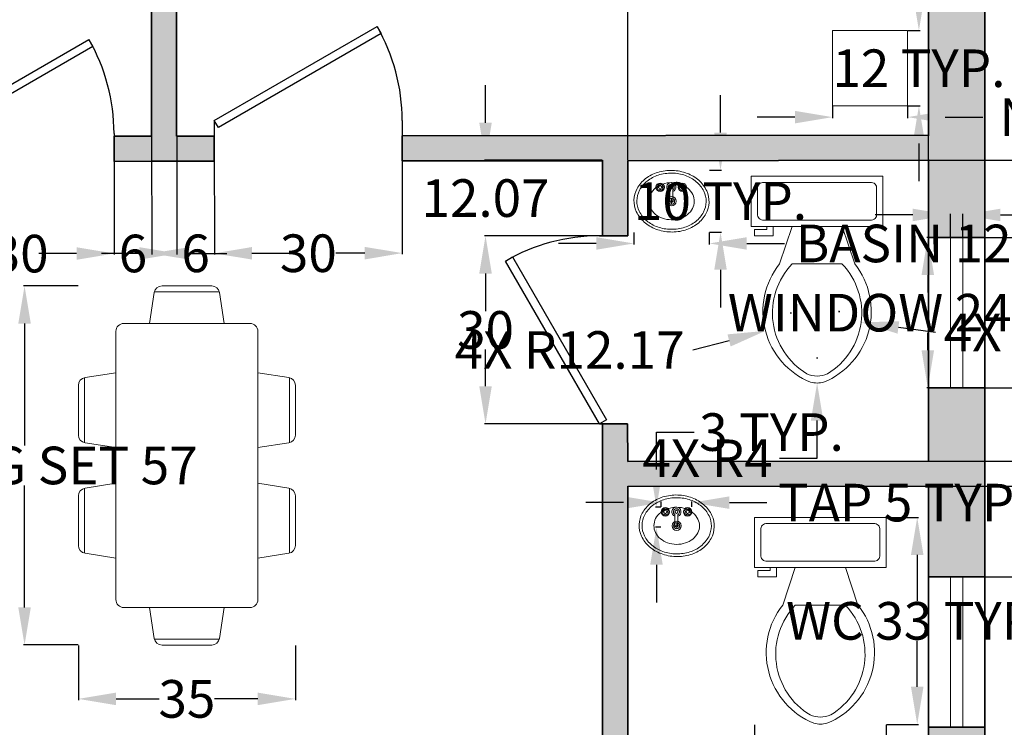
# Model space of a CAD drawing. Units: inches. Extents: x 98 to 487, y -240 to 141.
# Tile 3 of 5: x 251 to 408, y -81 to 32. Entities that reach past the tile are written whole.
import ezdxf

# ---------------------------------------------------------------- set-up
doc = ezdxf.new("R2010")
doc.units = ezdxf.units.IN
doc.header["$MEASUREMENT"] = 0
for name, color, linetype, lineweight in [('A-ANNO-DIMS', 2, 'Continuous', 18), ('A-DOOR', 3, 'Continuous', 25), ('A-FLOR-FIXT', 9, 'Continuous', 18), ('A-FURN', 8, 'Continuous', 18), ('A-GLAZ', 4, 'Continuous', 18), ('A-WALL', 7, 'Continuous', 35)]:
    doc.layers.add(name, color=color, linetype=linetype, lineweight=lineweight)
doc.layers.add('A-WALL-PATT', color=251, linetype='Continuous', lineweight=13, true_color=0x636466)
doc.styles.get("Standard").update_dxf_attribs({"font": 'arial.ttf'})
doc.dimstyles.get("Standard").update_dxf_attribs({"dimtxt": 6, "dimasz": 6, "dimexe": 0.18, "dimexo": 0.0625, "dimgap": 0.09, "dimtad": 0, "dimtih": 1, "dimtoh": 1, "dimdec": 0, "dimzin": 0, "dimdsep": 46, "dimlunit": 4, "dimtxsty": 'Standard', "dimcen": 0.09, "dimadec": 0, "dimazin": 0, "dimtfac": 1, "dimtdec": 0, "dimtofl": 0, "dimtmove": 0, "dimatfit": 3, "dimfxl": 1, "dimtolj": 1, "dimtzin": 0, "dimarcsym": 0})

# ---------------------------------------------------------------- blocks, each defined once
blk = doc.blocks.new('Sink - Oval top')
for p, q in [((-1, 0), (1, 0)), ((0, 1), (0, -1))]:
    blk.add_line(p, q)
for points in [[(-12.23, 0.39, 0.117634), (-11.46, -3.36, 0.104469), (-8.88, -6.8, 0.090016), (-5.08, -9.07, 0.08192), (-0.32, -10.02, 0.08192), (4.49, -9.38, 0.090016), (8.42, -7.36, 0.104469), (11.22, -4.09, 0.117634), (12.23, -0.39, 0.117634), (11.46, 3.36, 0.104469), (8.88, 6.8, 0.090016), (5.08, 9.07, 0.08192), (0.32, 10.02, 0.08192), (-4.49, 9.38, 0.090016), (-8.42, 7.36, 0.104469), (-11.22, 4.09, 0.117634)], [(-11.29, 0.16, 0.118622), (-10.52, -3.25, 0.104678), (-8.07, -6.36, 0.089562), (-4.54, -8.37, 0.081185), (-0.13, -9.15, 0.081185), (4.3, -8.49, 0.089562), (7.89, -6.58, 0.104678), (10.42, -3.55, 0.118622), (11.29, -0.16, 0.118622), (10.52, 3.25, 0.104678), (8.07, 6.36, 0.089562), (4.54, 8.37, 0.081185), (0.13, 9.15, 0.081185), (-4.3, 8.49, 0.089562), (-7.89, 6.58, 0.104678), (-10.42, 3.55, 0.118622)], [(-7.42, 0.08, 0.118283), (-6.91, -2.17, 0.104607), (-5.29, -4.21, 0.089718), (-2.97, -5.53, 0.081436), (-0.07, -6.04, 0.081436), (2.84, -5.59, 0.089718), (5.2, -4.33, 0.104607), (6.86, -2.32, 0.118283), (7.42, -0.08, 0.118283), (6.91, 2.17, 0.104607), (5.29, 4.21, 0.089718), (2.97, 5.53, 0.081436), (0.07, 6.04, 0.081436), (-2.84, 5.59, 0.089718), (-5.2, 4.33, 0.104607), (-6.86, 2.32, 0.118283)]]:
    blk.add_lwpolyline(points, format="xyb", close=True)
for radius in [1.5, 1]:
    blk.add_circle((0, 0), radius)
blk = doc.blocks.new('Faucet - Bathroom top')
for p, q in [((-4.107, 0.125), (-4.375, 0.125)), ((-3.75, 0.4788), (-3.75, 0.75)), ((-3.5, 0.482), (-3.5, 0.75)), ((-3.1461, 0.125), (-2.875, 0.125)), ((3.143, 0.125), (2.875, 0.125)), ((3.5, 0.4788), (3.5, 0.75)), ((3.75, 0.482), (3.75, 0.75)), ((4.1039, 0.125), (4.375, 0.125)), ((-4.1039, -0.125), (-4.375, -0.125)), ((-3.75, -0.4821), (-3.75, -0.75)), ((-3.5, -0.4789), (-3.5, -0.75)), ((-3.143, -0.125), (-2.875, -0.125)), ((-0.5, -0.8639), (-0.5, -4.5)), ((0.5, -4.5), (0.5, -0.8631)), ((3.1461, -0.125), (2.875, -0.125)), ((3.5, -0.4821), (3.5, -0.75)), ((3.75, -0.4789), (3.75, -0.75)), ((4.107, -0.125), (4.375, -0.125))]:
    blk.add_line(p, q)
for centre, radius in [((-3.625, 0), 1.375), ((-4.625, 0), 0.2795), ((-3.625, 0), 0.5), ((-3.625, 1), 0.2795), ((-2.625, 0), 0.2795), ((0, 0), 0.5), ((3.625, 0), 1.375), ((2.625, 0), 0.2795), ((3.625, 0), 0.5), ((3.625, 1), 0.2795), ((4.625, 0), 0.2795), ((-3.625, -1), 0.2795), ((3.625, -1), 0.2795)]:
    blk.add_circle(centre, radius)
for centre, radius, start, end in [((-3.625, 0), 1, 105.2407, 164.2093), ((-3.625, 0), 1, 16.44125, 74.07887), ((0, 0), 1.5, 289.6514, 250.3603), ((0, 0), 1, 300.3431, 239.7554), ((3.625, 0), 1, 106.12, 164.0884), ((3.625, 0), 1, 16.23422, 73.90469), ((-3.625, 0), 1, 196.2342, 253.9047), ((-3.625, 0), 1, 286.12, 344.0884), ((3.625, 0), 1, 196.4413, 254.0789), ((3.625, 0), 1, 285.2407, 344.2093), ((0, -4.5), 0.5, 180, 0)]:
    blk.add_arc(centre, radius, start, end)
blk = doc.blocks.new('Toilet - top')
for p, q in [((9.5, -6), (9.5, -2)), ((-10, -8.5), (-8, -8.5)), ((-10, -9.5), (-10, -8.5)), ((-8, -8.5), (-8, -8)), ((-7, -8), (-7, -9.5)), ((-4, -8), (-6, -14)), ((4, -8), (6, -14)), ((-7, -9.5), (-10, -9.5)), ((4, -14), (-4, -14))]:
    blk.add_line(p, q)
blk.add_lwpolyline([(10.5, -8), (10.5, 0), (-10.5, 0), (-10.5, -8)], close=True)
for points in [[(8.5, -1), (-8.5, -1)], [(-9.5, -2), (-9.5, -6)], [(-8.5, -7), (8.5, -7)]]:
    blk.add_lwpolyline(points)
for centre, radius, start, end in [((-8.62, -1.88), 0.884, 81.8699, 188.1301), ((8.62, -1.88), 0.884, 351.8699, 98.1301), ((-8.62, -6.12), 0.884, 171.8699, 278.1301), ((8.62, -6.12), 0.884, 261.8699, 8.1301), ((3.52, -21.58), 12.17, 141.4691, 247.9714), ((4.2, -21.82), 11.33, 136.3677, 238.9468), ((-3.52, -21.58), 12.17, 292.0284, 38.5307), ((-4.2, -21.82), 11.33, 301.053, 43.6321), ((0, -27.88), 4, 245.7318, 294.2682), ((0, -29), 4, 254.8605, 285.1395)]:
    blk.add_arc(centre, radius, start, end)
blk = doc.blocks.new('Dining Set - 36 x 72 in.')
for p, q in [((-20.29, 27.5), (-7.71, 27.5)), ((7.71, 27.5), (20.29, 27.5)), ((-22.26, 25.81), (-23.48, 18)), ((-22.23, 26), (-5.76, 26)), ((-4.52, 18), (-5.74, 25.81)), ((5.74, 25.81), (4.52, 18)), ((5.77, 26), (22.24, 26)), ((23.48, 18), (22.26, 25.81)), ((34, 18), (-34, 18)), ((-36, 16), (-36, -16)), ((36, -16), (36, 16)), ((-44, 8.23), (-44, -8.24)), ((-43.81, 8.26), (-36, 9.48)), ((43.81, 8.26), (36, 9.48)), ((44, 8.23), (44, -8.24)), ((-45.5, 6.29), (-45.5, -6.29)), ((45.5, 6.29), (45.5, -6.29)), ((-36, -9.48), (-43.81, -8.26)), ((36, -9.48), (43.81, -8.26)), ((-34, -18), (34, -18)), ((-22.26, -25.81), (-23.48, -18)), ((-4.52, -18), (-5.74, -25.81)), ((5.74, -25.81), (4.52, -18)), ((23.48, -18), (22.26, -25.81)), ((-22.23, -26), (-5.76, -26)), ((5.77, -26), (22.24, -26)), ((-20.29, -27.5), (-7.71, -27.5)), ((7.71, -27.5), (20.29, -27.5))]:
    blk.add_line(p, q)
for centre, start, end in [((-20.29, 25.5), 90, 171.1198), ((-7.71, 25.5), 8.881, 90), ((7.71, 25.5), 90, 171.1198), ((20.29, 25.5), 8.881, 90), ((-34, 16), 90, 180), ((34, 16), 0, 90), ((-43.5, 6.29), 98.8806, 180), ((43.5, 6.29), 0, 81.1194), ((-43.5, -6.29), 180, 261.1194), ((43.5, -6.29), 278.8806, 0), ((-34, -16), 180, 270), ((34, -16), 270, 0), ((-20.29, -25.5), 188.8802, 270), ((-7.71, -25.5), 270, 351.1191), ((7.71, -25.5), 188.8802, 270), ((20.29, -25.5), 270, 351.1191)]:
    blk.add_arc(centre, 2, start, end)
blk = doc.blocks.new('*U8')
for p, q in [((0, 0), (0, -6)), ((40, 0), (40, -6))]:
    blk.add_line(p, q)
blk.add_lwpolyline([(0, 0), (34.64, 20), (35.52, 18.48), (0.87, -1.52)], close=True)
blk.add_arc((0, 0), 40, 0, 30)
blk = doc.blocks.new('GLAZ-24IN')
for p, q in [((0, 24), (0, 0)), ((2, 24), (2, 0))]:
    blk.add_line(p, q)
blk = doc.blocks.new('NIGHTSTAND-12IN-SQUARE')
blk.add_lwpolyline([(12, 12), (0, 12), (0, 0), (12, 0)], close=True)
blk = doc.blocks.new('*D26')
at = {"layer": 'A-ANNO-DIMS', "color": 0, "lineweight": -2, "transparency": 16777216}
for p, q in [((380.45, 18.25), (380.45, 16.33)), ((392.45, 18.25), (392.45, 16.33)), ((374.45, 16.51), (368.45, 16.51)), ((398.45, 16.51), (404.45, 16.51))]:
    blk.add_line(p, q, dxfattribs=at)
at = {"layer": 'A-ANNO-DIMS', "color": 0, "transparency": 16777216}
for points in [[(374.45, 17.51), (374.45, 15.51), (380.45, 16.51)], [(398.45, 17.51), (398.45, 15.51), (392.45, 16.51)]]:
    blk.add_solid(points, dxfattribs=at)
at = {"layer": 'Defpoints', "color": 0, "transparency": 16777216}
for p in [(380.45, 18.31), (392.45, 18.31), (392.45, 16.51)]:
    blk.add_point(p, dxfattribs=at)
at = {"layer": 'A-ANNO-DIMS', "color": 0, "transparency": 16777216, "insert": (447.4, 16.51), "char_height": 6, "attachment_point": 5}
blk.add_mtext('\\A1;NIGHTSTAND 12 TYP.', dxfattribs=at)
blk = doc.blocks.new('*D27')
at = {"layer": 'A-ANNO-DIMS', "color": 0, "lineweight": -2, "transparency": 16777216}
for p, q in [((394.25, 36.31), (394.25, 42.31)), ((392.51, 30.31), (394.43, 30.31)), ((392.51, 18.31), (394.43, 18.31)), ((394.25, 12.31), (394.25, 6.31))]:
    blk.add_line(p, q, dxfattribs=at)
at = {"layer": 'A-ANNO-DIMS', "color": 0, "transparency": 16777216}
for points in [[(393.25, 36.31), (395.25, 36.31), (394.25, 30.31)], [(393.25, 12.31), (395.25, 12.31), (394.25, 18.31)]]:
    blk.add_solid(points, dxfattribs=at)
at = {"layer": 'Defpoints', "color": 0, "transparency": 16777216}
for p in [(392.45, 30.31), (394.25, 30.31), (392.45, 18.31)]:
    blk.add_point(p, dxfattribs=at)
at = {"layer": 'A-ANNO-DIMS', "color": 0, "transparency": 16777216, "insert": (394.25, 24.31), "char_height": 6, "attachment_point": 5}
blk.add_mtext('\\A1;12 TYP.', dxfattribs=at)
blk = doc.blocks.new('*D30')
at = {"layer": 'A-ANNO-DIMS', "color": 0, "lineweight": -2, "transparency": 16777216}
for p, q in [((399.2, -2.7), (395.49, -2.7)), ((395.67, -8.7), (395.67, -11.5)), ((395.67, -20.7), (395.67, -17.89)), ((399.2, -26.7), (395.49, -26.7))]:
    blk.add_line(p, q, dxfattribs=at)
at = {"layer": 'A-ANNO-DIMS', "color": 0, "transparency": 16777216}
for points in [[(394.67, -8.7), (396.67, -8.7), (395.67, -2.7)], [(394.67, -20.7), (396.67, -20.7), (395.67, -26.7)]]:
    blk.add_solid(points, dxfattribs=at)
at = {"layer": 'Defpoints', "color": 0, "transparency": 16777216}
for p in [(395.67, -2.7), (399.27, -2.7), (399.27, -26.7)]:
    blk.add_point(p, dxfattribs=at)
at = {"layer": 'A-ANNO-DIMS', "color": 0, "transparency": 16777216, "insert": (395.67, -14.7), "char_height": 6, "attachment_point": 5}
blk.add_mtext('\\A1;WINDOW 24 TYP.', dxfattribs=at)
blk = doc.blocks.new('*D31')
at = {"layer": 'A-ANNO-DIMS', "color": 0, "lineweight": -2, "transparency": 16777216}
for p, q in [((393.27, 0.9), (387.27, 0.9)), ((399.27, -2.64), (399.27, 1.08)), ((401.27, -2.64), (401.27, 1.08)), ((407.27, 0.9), (413.27, 0.9))]:
    blk.add_line(p, q, dxfattribs=at)
at = {"layer": 'A-ANNO-DIMS', "color": 0, "transparency": 16777216}
for points in [[(393.27, 1.9), (393.27, -0.1), (399.27, 0.9)], [(407.27, 1.9), (407.27, -0.1), (401.27, 0.9)]]:
    blk.add_solid(points, dxfattribs=at)
at = {"layer": 'Defpoints', "color": 0, "transparency": 16777216}
for p in [(401.27, 0.9), (399.27, -2.7), (401.27, -2.7)]:
    blk.add_point(p, dxfattribs=at)
at = {"layer": 'A-ANNO-DIMS', "color": 0, "transparency": 16777216, "insert": (425.68, 0.9), "char_height": 6, "attachment_point": 5}
blk.add_mtext('\\A1;2 TYP.', dxfattribs=at)
blk = doc.blocks.new('*D32')
at = {"layer": 'A-ANNO-DIMS', "color": 0, "lineweight": -2, "transparency": 16777216}
for p, q in [((348.74, -1.91), (348.74, -3.83)), ((360.78, -1.91), (360.78, -3.83)), ((342.74, -3.65), (336.74, -3.65)), ((366.78, -3.65), (372.78, -3.65))]:
    blk.add_line(p, q, dxfattribs=at)
at = {"layer": 'A-ANNO-DIMS', "color": 0, "transparency": 16777216}
for points in [[(342.74, -2.65), (342.74, -4.65), (348.74, -3.65)], [(366.78, -2.65), (366.78, -4.65), (360.78, -3.65)]]:
    blk.add_solid(points, dxfattribs=at)
at = {"layer": 'Defpoints', "color": 0, "transparency": 16777216}
for p in [(348.74, -1.85), (360.78, -1.85), (360.78, -3.65)]:
    blk.add_point(p, dxfattribs=at)
at = {"layer": 'A-ANNO-DIMS', "color": 0, "transparency": 16777216, "insert": (401.08, -3.65), "char_height": 6, "attachment_point": 5}
blk.add_mtext('\\A1;BASIN 12 TYP.', dxfattribs=at)
blk = doc.blocks.new('*D33')
at = {"layer": 'A-ANNO-DIMS', "color": 0, "lineweight": -2, "transparency": 16777216}
for p, q in [((362.58, 14.03), (362.58, 20.03)), ((360.84, 8.03), (362.76, 8.03)), ((360.84, -1.85), (362.76, -1.85)), ((362.58, -7.85), (362.58, -13.85))]:
    blk.add_line(p, q, dxfattribs=at)
at = {"layer": 'A-ANNO-DIMS', "color": 0, "transparency": 16777216}
for points in [[(361.58, 14.03), (363.58, 14.03), (362.58, 8.03)], [(361.58, -7.85), (363.58, -7.85), (362.58, -1.85)]]:
    blk.add_solid(points, dxfattribs=at)
at = {"layer": 'Defpoints', "color": 0, "transparency": 16777216}
for p in [(360.78, 8.03), (362.58, 8.03), (360.78, -1.85)]:
    blk.add_point(p, dxfattribs=at)
at = {"layer": 'A-ANNO-DIMS', "color": 0, "transparency": 16777216, "insert": (362.58, 3.09), "char_height": 6, "attachment_point": 5}
blk.add_mtext('\\A1;10 TYP.', dxfattribs=at)
blk = doc.blocks.new('*D34')
at = {"layer": 'A-ANNO-DIMS', "color": 0, "lineweight": -2, "transparency": 16777216}
for p, q in [((347.1, -45.01), (341.1, -45.01)), ((353.1, -45.68), (353.1, -44.83)), ((358, -45.68), (358, -44.83)), ((364, -45.01), (370, -45.01))]:
    blk.add_line(p, q, dxfattribs=at)
at = {"layer": 'A-ANNO-DIMS', "color": 0, "transparency": 16777216}
for points in [[(347.1, -44.01), (347.1, -46.01), (353.1, -45.01)], [(364, -44.01), (364, -46.01), (358, -45.01)]]:
    blk.add_solid(points, dxfattribs=at)
at = {"layer": 'Defpoints', "color": 0, "transparency": 16777216}
for p in [(358, -45.01), (353.1, -45.75), (358, -45.75)]:
    blk.add_point(p, dxfattribs=at)
at = {"layer": 'A-ANNO-DIMS', "color": 0, "transparency": 16777216, "insert": (391.75, -45.01), "char_height": 6, "attachment_point": 5}
blk.add_mtext('\\A1;TAP 5 TYP.', dxfattribs=at)
blk = doc.blocks.new('*D35')
at = {"layer": 'A-ANNO-DIMS', "color": 0, "lineweight": -2, "transparency": 16777216}
for p, q in [((352.36, -39.75), (352.36, -33.75)), ((352.36, -33.75), (358.36, -33.75)), ((353.03, -45.75), (352.18, -45.75)), ((353.03, -48.93), (352.18, -48.93)), ((352.36, -54.93), (352.36, -60.93))]:
    blk.add_line(p, q, dxfattribs=at)
at = {"layer": 'A-ANNO-DIMS', "color": 0, "transparency": 16777216}
for points in [[(351.36, -39.75), (353.36, -39.75), (352.36, -45.75)], [(351.36, -54.93), (353.36, -54.93), (352.36, -48.93)]]:
    blk.add_solid(points, dxfattribs=at)
at = {"layer": 'Defpoints', "color": 0, "transparency": 16777216}
for p in [(352.36, -45.75), (353.1, -45.75), (353.1, -48.93)]:
    blk.add_point(p, dxfattribs=at)
at = {"layer": 'A-ANNO-DIMS', "color": 0, "transparency": 16777216, "insert": (370.72, -33.75), "char_height": 6, "attachment_point": 5}
blk.add_mtext('\\A1;3 TYP.', dxfattribs=at)
blk = doc.blocks.new('*D36')
at = {"layer": 'A-ANNO-DIMS', "color": 0, "lineweight": -2, "transparency": 16777216}
for p, q in [((389.08, -47.36), (394.16, -47.36)), ((393.98, -53.36), (393.98, -60.69)), ((393.98, -74.4), (393.98, -67.08)), ((389.08, -80.4), (394.16, -80.4))]:
    blk.add_line(p, q, dxfattribs=at)
at = {"layer": 'A-ANNO-DIMS', "color": 0, "transparency": 16777216}
for points in [[(392.98, -53.36), (394.98, -53.36), (393.98, -47.36)], [(392.98, -74.4), (394.98, -74.4), (393.98, -80.4)]]:
    blk.add_solid(points, dxfattribs=at)
at = {"layer": 'Defpoints', "color": 0, "transparency": 16777216}
for p in [(389.02, -47.36), (393.98, -47.36), (389.02, -80.4)]:
    blk.add_point(p, dxfattribs=at)
at = {"layer": 'A-ANNO-DIMS', "color": 0, "transparency": 16777216, "insert": (393.98, -63.88), "char_height": 6, "attachment_point": 5}
blk.add_mtext('\\A1;WC 33 TYP.', dxfattribs=at)
blk = doc.blocks.new('*D37')
at = {"layer": 'A-ANNO-DIMS', "color": 0, "lineweight": -2, "transparency": 16777216}
for p, q in [((368.02, -80.47), (368.02, -85.54)), ((389.02, -80.47), (389.02, -85.54)), ((374.02, -85.36), (383.02, -85.36)), ((389.02, -85.36), (395.02, -85.36))]:
    blk.add_line(p, q, dxfattribs=at)
at = {"layer": 'A-ANNO-DIMS', "color": 0, "transparency": 16777216}
for points in [[(374.02, -84.36), (374.02, -86.36), (368.02, -85.36)], [(383.02, -84.36), (383.02, -86.36), (389.02, -85.36)]]:
    blk.add_solid(points, dxfattribs=at)
at = {"layer": 'Defpoints', "color": 0, "transparency": 16777216}
for p in [(368.02, -80.4), (389.02, -80.4), (389.02, -85.36)]:
    blk.add_point(p, dxfattribs=at)
at = {"layer": 'A-ANNO-DIMS', "color": 0, "transparency": 16777216, "insert": (409.76, -85.36), "char_height": 6, "attachment_point": 5}
blk.add_mtext('\\A1;21 TYP.', dxfattribs=at)
blk = doc.blocks.new('*D38')
at = {"layer": 'A-ANNO-DIMS', "color": 0, "lineweight": -2, "transparency": 16777216}
for p, q in [((260.02, -10.43), (251.31, -10.43)), ((251.49, -16.43), (251.49, -35.89)), ((251.49, -61.73), (251.49, -42.27)), ((260.02, -67.73), (251.31, -67.73))]:
    blk.add_line(p, q, dxfattribs=at)
at = {"layer": 'A-ANNO-DIMS', "color": 0, "transparency": 16777216}
for points in [[(250.49, -16.43), (252.49, -16.43), (251.49, -10.43)], [(250.49, -61.73), (252.49, -61.73), (251.49, -67.73)]]:
    blk.add_solid(points, dxfattribs=at)
at = {"layer": 'Defpoints', "color": 0, "transparency": 16777216}
for p in [(260.09, -10.43), (251.49, -67.73), (260.09, -67.73)]:
    blk.add_point(p, dxfattribs=at)
at = {"layer": 'A-ANNO-DIMS', "color": 0, "transparency": 16777216, "insert": (251.49, -39.08), "char_height": 6, "attachment_point": 5}
blk.add_mtext('\\A1;DINING SET 57', dxfattribs=at)
blk = doc.blocks.new('*D39')
at = {"layer": 'A-ANNO-DIMS', "color": 0, "lineweight": -2, "transparency": 16777216}
for p, q in [((260.09, -67.8), (260.09, -76.51)), ((294.72, -67.8), (294.72, -76.51)), ((266.09, -76.33), (273, -76.33)), ((288.72, -76.33), (281.81, -76.33))]:
    blk.add_line(p, q, dxfattribs=at)
at = {"layer": 'A-ANNO-DIMS', "color": 0, "transparency": 16777216}
for points in [[(266.09, -75.33), (266.09, -77.33), (260.09, -76.33)], [(288.72, -75.33), (288.72, -77.33), (294.72, -76.33)]]:
    blk.add_solid(points, dxfattribs=at)
at = {"layer": 'Defpoints', "color": 0, "transparency": 16777216}
for p in [(260.09, -67.73), (294.72, -67.73), (294.72, -76.33)]:
    blk.add_point(p, dxfattribs=at)
at = {"layer": 'A-ANNO-DIMS', "color": 0, "transparency": 16777216, "insert": (277.4, -76.33), "char_height": 6, "attachment_point": 5}
blk.add_mtext('\\A1;35', dxfattribs=at)
blk = doc.blocks.new('*D47')
at = {"layer": 'A-ANNO-DIMS', "color": 0, "lineweight": -2, "transparency": 16777216}
for p, q in [((404.83, 118.64), (423.65, 118.64)), ((423.47, 112.64), (423.47, -46.22)), ((423.47, -211.38), (423.47, -52.53)), ((404.83, -217.38), (423.65, -217.38))]:
    blk.add_line(p, q, dxfattribs=at)
at = {"layer": 'A-ANNO-DIMS', "color": 0, "transparency": 16777216}
for points in [[(422.47, 112.64), (424.47, 112.64), (423.47, 118.64)], [(422.47, -211.38), (424.47, -211.38), (423.47, -217.38)]]:
    blk.add_solid(points, dxfattribs=at)
at = {"layer": 'Defpoints', "color": 0, "transparency": 16777216}
for p in [(404.77, 118.64), (404.77, -217.38), (423.47, -217.38)]:
    blk.add_point(p, dxfattribs=at)
at = {"layer": 'A-ANNO-DIMS', "color": 0, "transparency": 16777216, "insert": (423.47, -49.37), "char_height": 6, "attachment_point": 5}
blk.add_mtext('\\A1;336', dxfattribs=at)
blk = doc.blocks.new('*D65')
at = {"layer": 'A-ANNO-DIMS', "color": 0, "lineweight": -2, "transparency": 16777216}
for p, q in [((395.83, 9.62), (414.65, 9.62)), ((414.47, 3.62), (414.47, -11.22)), ((414.47, -32.38), (414.47, -17.53)), ((395.83, -38.38), (414.65, -38.38))]:
    blk.add_line(p, q, dxfattribs=at)
at = {"layer": 'A-ANNO-DIMS', "color": 0, "transparency": 16777216}
for points in [[(413.47, 3.62), (415.47, 3.62), (414.47, 9.62)], [(413.47, -32.38), (415.47, -32.38), (414.47, -38.38)]]:
    blk.add_solid(points, dxfattribs=at)
at = {"layer": 'Defpoints', "color": 0, "transparency": 16777216}
for p in [(395.77, 9.62), (395.77, -38.38), (414.47, -38.38)]:
    blk.add_point(p, dxfattribs=at)
at = {"layer": 'A-ANNO-DIMS', "color": 0, "transparency": 16777216, "insert": (414.47, -14.38), "char_height": 6, "attachment_point": 5}
blk.add_mtext('\\A1;48', dxfattribs=at)
blk = doc.blocks.new('*D66')
at = {"layer": 'A-ANNO-DIMS', "color": 0, "lineweight": -2, "transparency": 16777216}
for p, q in [((395.83, -42.38), (414.65, -42.38)), ((414.47, -48.38), (414.47, -63.22)), ((414.47, -84.38), (414.47, -69.53)), ((395.83, -90.38), (414.65, -90.38))]:
    blk.add_line(p, q, dxfattribs=at)
at = {"layer": 'A-ANNO-DIMS', "color": 0, "transparency": 16777216}
for points in [[(413.47, -48.38), (415.47, -48.38), (414.47, -42.38)], [(413.47, -84.38), (415.47, -84.38), (414.47, -90.38)]]:
    blk.add_solid(points, dxfattribs=at)
at = {"layer": 'Defpoints', "color": 0, "transparency": 16777216}
for p in [(395.77, -42.38), (395.77, -90.38), (414.47, -90.38)]:
    blk.add_point(p, dxfattribs=at)
at = {"layer": 'A-ANNO-DIMS', "color": 0, "transparency": 16777216, "insert": (414.47, -66.38), "char_height": 6, "attachment_point": 5}
blk.add_mtext('\\A1;48', dxfattribs=at)
blk = doc.blocks.new('*D67')
at = {"layer": 'A-ANNO-DIMS', "color": 0, "lineweight": -2, "transparency": 16777216}
for p, q in [((347.77, 9.62), (347.77, 137.52)), ((353.77, 137.34), (367.25, 137.34)), ((389.77, 137.34), (376.28, 137.34)), ((395.77, 9.69), (395.77, 137.52))]:
    blk.add_line(p, q, dxfattribs=at)
at = {"layer": 'A-ANNO-DIMS', "color": 0, "transparency": 16777216}
for points in [[(353.77, 138.34), (353.77, 136.34), (347.77, 137.34)], [(389.77, 138.34), (389.77, 136.34), (395.77, 137.34)]]:
    blk.add_solid(points, dxfattribs=at)
at = {"layer": 'Defpoints', "color": 0, "transparency": 16777216}
for p in [(395.77, 137.34), (347.77, 9.56), (395.77, 9.62)]:
    blk.add_point(p, dxfattribs=at)
at = {"layer": 'A-ANNO-DIMS', "color": 0, "transparency": 16777216, "insert": (371.77, 137.34), "char_height": 6, "attachment_point": 5}
blk.add_mtext('\\A1;48', dxfattribs=at)
blk = doc.blocks.new('*D70')
at = {"layer": 'A-ANNO-DIMS', "color": 0, "lineweight": -2, "transparency": 16777216}
for p, q in [((343.7, -2.45), (324.89, -2.45)), ((325.07, -8.45), (325.07, -14.29)), ((325.07, -26.45), (325.07, -20.6)), ((343.7, -32.45), (324.89, -32.45))]:
    blk.add_line(p, q, dxfattribs=at)
at = {"layer": 'A-ANNO-DIMS', "color": 0, "transparency": 16777216}
for points in [[(324.07, -8.45), (326.07, -8.45), (325.07, -2.45)], [(324.07, -26.45), (326.07, -26.45), (325.07, -32.45)]]:
    blk.add_solid(points, dxfattribs=at)
at = {"layer": 'Defpoints', "color": 0, "transparency": 16777216}
for p in [(325.07, -2.45), (343.77, -2.45), (343.77, -32.45)]:
    blk.add_point(p, dxfattribs=at)
at = {"layer": 'A-ANNO-DIMS', "color": 0, "transparency": 16777216, "insert": (325.07, -17.45), "char_height": 6, "attachment_point": 5}
blk.add_mtext('\\A1;30', dxfattribs=at)
blk = doc.blocks.new('*D71')
at = {"layer": 'A-ANNO-DIMS', "color": 0, "lineweight": -2, "transparency": 16777216}
for p, q in [((235.77, 13.35), (235.79, -5.47)), ((265.77, 13.39), (265.79, -5.43)), ((241.79, -5.28), (246.42, -5.28)), ((259.79, -5.26), (255.17, -5.26))]:
    blk.add_line(p, q, dxfattribs=at)
at = {"layer": 'A-ANNO-DIMS', "color": 0, "transparency": 16777216}
for points in [[(241.79, -4.28), (241.79, -6.28), (235.79, -5.29)], [(259.79, -4.26), (259.79, -6.26), (265.79, -5.25)]]:
    blk.add_solid(points, dxfattribs=at)
at = {"layer": 'Defpoints', "color": 0, "transparency": 16777216}
for p in [(235.77, 13.41), (265.77, 13.45), (235.79, -5.29)]:
    blk.add_point(p, dxfattribs=at)
at = {"layer": 'A-ANNO-DIMS', "color": 0, "transparency": 16777216, "insert": (250.79, -5.27), "char_height": 6, "attachment_point": 5}
blk.add_mtext('\\A1;30', dxfattribs=at)
blk = doc.blocks.new('*D72')
at = {"layer": 'A-ANNO-DIMS', "color": 0, "lineweight": -2, "transparency": 16777216}
for p, q in [((265.77, 13.39), (265.79, -5.43)), ((271.77, 13.4), (271.79, -5.42)), ((259.79, -5.26), (253.79, -5.27)), ((277.79, -5.23), (283.79, -5.23))]:
    blk.add_line(p, q, dxfattribs=at)
at = {"layer": 'A-ANNO-DIMS', "color": 0, "transparency": 16777216}
for points in [[(259.79, -4.26), (259.79, -6.26), (265.79, -5.25)], [(277.79, -4.23), (277.79, -6.23), (271.79, -5.24)]]:
    blk.add_solid(points, dxfattribs=at)
at = {"layer": 'Defpoints', "color": 0, "transparency": 16777216}
for p in [(265.77, 13.45), (271.77, 13.46), (265.79, -5.25)]:
    blk.add_point(p, dxfattribs=at)
at = {"layer": 'A-ANNO-DIMS', "color": 0, "transparency": 16777216, "insert": (268.79, -5.25), "char_height": 6, "attachment_point": 5}
blk.add_mtext('\\A1;6', dxfattribs=at)
blk = doc.blocks.new('*D73')
at = {"layer": 'A-ANNO-DIMS', "color": 0, "lineweight": -2, "transparency": 16777216}
for p, q in [((275.77, 13.4), (275.79, -5.42)), ((281.77, 13.41), (281.79, -5.41)), ((269.79, -5.24), (263.79, -5.25)), ((287.79, -5.22), (293.79, -5.21))]:
    blk.add_line(p, q, dxfattribs=at)
at = {"layer": 'A-ANNO-DIMS', "color": 0, "transparency": 16777216}
for points in [[(269.79, -4.24), (269.79, -6.24), (275.79, -5.24)], [(287.79, -4.22), (287.79, -6.22), (281.79, -5.23)]]:
    blk.add_solid(points, dxfattribs=at)
at = {"layer": 'Defpoints', "color": 0, "transparency": 16777216}
for p in [(275.77, 13.46), (281.77, 13.47), (275.79, -5.24)]:
    blk.add_point(p, dxfattribs=at)
at = {"layer": 'A-ANNO-DIMS', "color": 0, "transparency": 16777216, "insert": (278.79, -5.23), "char_height": 6, "attachment_point": 5}
blk.add_mtext('\\A1;6', dxfattribs=at)
blk = doc.blocks.new('*D74')
at = {"layer": 'A-ANNO-DIMS', "color": 0, "lineweight": -2, "transparency": 16777216}
for p, q in [((281.77, 13.41), (281.79, -5.41)), ((311.77, 13.45), (311.79, -5.37)), ((287.79, -5.22), (292.42, -5.21)), ((305.79, -5.2), (301.17, -5.2))]:
    blk.add_line(p, q, dxfattribs=at)
at = {"layer": 'A-ANNO-DIMS', "color": 0, "transparency": 16777216}
for points in [[(287.79, -4.22), (287.79, -6.22), (281.79, -5.23)], [(305.79, -4.2), (305.79, -6.2), (311.79, -5.19)]]:
    blk.add_solid(points, dxfattribs=at)
at = {"layer": 'Defpoints', "color": 0, "transparency": 16777216}
for p in [(281.77, 13.47), (311.77, 13.51), (281.79, -5.23)]:
    blk.add_point(p, dxfattribs=at)
at = {"layer": 'A-ANNO-DIMS', "color": 0, "transparency": 16777216, "insert": (296.79, -5.21), "char_height": 6, "attachment_point": 5}
blk.add_mtext('\\A1;30', dxfattribs=at)
blk = doc.blocks.new('*D75')
at = {"layer": 'A-ANNO-DIMS', "color": 0, "lineweight": -2, "transparency": 16777216}
for p, q in [((325.07, 15.62), (325.07, 21.62)), ((343.7, 9.62), (324.89, 9.62)), ((343.7, -2.45), (324.89, -2.45)), ((325.07, -8.45), (325.07, -14.45))]:
    blk.add_line(p, q, dxfattribs=at)
at = {"layer": 'A-ANNO-DIMS', "color": 0, "transparency": 16777216}
for points in [[(324.07, 15.62), (326.07, 15.62), (325.07, 9.62)], [(324.07, -8.45), (326.07, -8.45), (325.07, -2.45)]]:
    blk.add_solid(points, dxfattribs=at)
at = {"layer": 'Defpoints', "color": 0, "transparency": 16777216}
for p in [(325.07, 9.62), (343.77, 9.62), (343.77, -2.45)]:
    blk.add_point(p, dxfattribs=at)
at = {"layer": 'A-ANNO-DIMS', "color": 0, "transparency": 16777216, "insert": (325.07, 3.59), "char_height": 6, "attachment_point": 5}
blk.add_mtext('\\A1;12.07', dxfattribs=at)
blk = doc.blocks.new('*D76')
at = {"layer": 'A-ANNO-DIMS', "color": 0, "lineweight": -2, "transparency": 16777216}
for p, q in [((404.83, -26.7), (423.65, -26.7)), ((423.47, -32.7), (423.47, -38.63)), ((423.47, -50.87), (423.47, -44.94)), ((404.83, -56.87), (423.65, -56.87))]:
    blk.add_line(p, q, dxfattribs=at)
at = {"layer": 'A-ANNO-DIMS', "color": 0, "transparency": 16777216}
for points in [[(422.47, -32.7), (424.47, -32.7), (423.47, -26.7)], [(422.47, -50.87), (424.47, -50.87), (423.47, -56.87)]]:
    blk.add_solid(points, dxfattribs=at)
at = {"layer": 'Defpoints', "color": 0, "transparency": 16777216}
for p in [(404.77, -26.7), (404.77, -56.87), (423.47, -56.87)]:
    blk.add_point(p, dxfattribs=at)
at = {"layer": 'A-ANNO-DIMS', "color": 0, "transparency": 16777216, "insert": (423.47, -41.78), "char_height": 6, "attachment_point": 5}
blk.add_mtext('\\A1;30.17', dxfattribs=at)
blk = doc.blocks.new('*D77')
at = {"layer": 'A-ANNO-DIMS', "color": 0, "lineweight": -2, "transparency": 16777216}
for p, q in [((423.47, 9.62), (423.47, 15.62)), ((423.47, 15.62), (429.47, 15.62)), ((395.83, 9.62), (423.65, 9.62)), ((423.47, 3.3), (423.47, 3.62)), ((404.83, -2.7), (423.65, -2.7))]:
    blk.add_line(p, q, dxfattribs=at)
at = {"layer": 'A-ANNO-DIMS', "color": 0, "transparency": 16777216}
for points in [[(422.47, 3.62), (424.47, 3.62), (423.47, 9.62)], [(422.47, 3.3), (424.47, 3.3), (423.47, -2.7)]]:
    blk.add_solid(points, dxfattribs=at)
at = {"layer": 'Defpoints', "color": 0, "transparency": 16777216}
for p in [(395.77, 9.62), (423.47, 9.62), (404.77, -2.7)]:
    blk.add_point(p, dxfattribs=at)
at = {"layer": 'A-ANNO-DIMS', "color": 0, "transparency": 16777216, "insert": (439.37, 15.62), "char_height": 6, "attachment_point": 5}
blk.add_mtext('\\A1;12.32', dxfattribs=at)
blk = doc.blocks.new('*D84')
at = {"layer": 'A-ANNO-DIMS', "color": 0, "lineweight": -2, "transparency": 16777216}
for p, q in [((381.43, -14.51), (381.61, -14.51)), ((381.52, -14.6), (381.52, -14.42)), ((358.14, -20.65), (363.95, -19.12))]:
    blk.add_line(p, q, dxfattribs=at)
at = {"layer": 'A-ANNO-DIMS', "color": 0, "transparency": 16777216}
blk.add_solid([(363.69, -18.16), (364.2, -20.09), (369.75, -17.6)], dxfattribs=at)
at = {"layer": 'Defpoints', "color": 0, "transparency": 16777216}
for p in [(381.52, -14.51), (369.75, -17.6)]:
    blk.add_point(p, dxfattribs=at)
at = {"layer": 'A-ANNO-DIMS', "color": 0, "transparency": 16777216, "insert": (338.49, -20.65), "char_height": 6, "attachment_point": 5}
blk.add_mtext('\\A1;4X R12.17', dxfattribs=at)
blk = doc.blocks.new('*D85')
at = {"layer": 'A-ANNO-DIMS', "color": 0, "lineweight": -2, "transparency": 16777216}
for p, q in [((373.71, -14.74), (373.89, -14.74)), ((373.8, -14.83), (373.8, -14.65)), ((396.92, -17.85), (390.97, -17.05))]:
    blk.add_line(p, q, dxfattribs=at)
at = {"layer": 'A-ANNO-DIMS', "color": 0, "transparency": 16777216}
blk.add_solid([(391.11, -16.06), (390.84, -18.04), (385.03, -16.25)], dxfattribs=at)
at = {"layer": 'Defpoints', "color": 0, "transparency": 16777216}
for p in [(373.8, -14.74), (385.03, -16.25)]:
    blk.add_point(p, dxfattribs=at)
at = {"layer": 'A-ANNO-DIMS', "color": 0, "transparency": 16777216, "insert": (416.57, -17.85), "char_height": 6, "attachment_point": 5}
blk.add_mtext('\\A1;4X R11.33', dxfattribs=at)
blk = doc.blocks.new('*D86')
at = {"layer": 'A-ANNO-DIMS', "color": 0, "lineweight": -2, "transparency": 16777216}
for p, q in [((377.91, -21.93), (378.09, -21.93)), ((378, -22.02), (378, -21.84)), ((378, -37.93), (378, -31.93)), ((372, -37.93), (378, -37.93))]:
    blk.add_line(p, q, dxfattribs=at)
at = {"layer": 'A-ANNO-DIMS', "color": 0, "transparency": 16777216}
blk.add_solid([(377, -31.93), (379, -31.93), (378, -25.93)], dxfattribs=at)
at = {"layer": 'Defpoints', "color": 0, "transparency": 16777216}
for p in [(378, -21.93), (378, -25.93)]:
    blk.add_point(p, dxfattribs=at)
at = {"layer": 'A-ANNO-DIMS', "color": 0, "transparency": 16777216, "insert": (360.51, -37.93), "char_height": 6, "attachment_point": 5}
blk.add_mtext('\\A1;4X R4', dxfattribs=at)

msp = doc.modelspace()

# ---------------------------------------------------------------- hatches: boundary and pattern name
at = {"layer": 'A-WALL-PATT'}
h = msp.add_hatch(color=256, dxfattribs=at)
h.dxf.hatch_style = 1
h.paths.add_polyline_path([(316.6174, 118.5177), (214.5584, 118.3815), (214.5584, 109.3815), (271.7663, 109.4578), (271.7663, 13.4577), (265.7717, 13.4497), (265.7717, 9.4497), (271.7663, 9.4577), (281.7716, 9.4711), (281.7663, 13.4711), (275.7663, 13.4631), (275.7663, 109.4632), (316.6174, 109.5177)])
h = msp.add_hatch(color=256, dxfattribs=at)
h.dxf.hatch_style = 1
h.paths.add_polyline_path([(404.7663, 118.6353), (364.6174, 118.5817), (364.6174, 109.5817), (395.7663, 109.6233), (395.7663, 13.6232), (311.7663, 13.5111), (311.7716, 9.5111), (343.7663, 9.5538), (343.7663, -2.4462), (347.7663, -2.4409), (347.7663, 9.5591), (395.7663, 9.6232), (395.7663, -2.698), (404.7663, -2.698)])
h = msp.add_hatch(color=256, dxfattribs=at)
h.dxf.hatch_style = 1
h.paths.add_polyline_path([(404.7663, -26.698), (395.7663, -26.698), (395.7663, -38.3769), (347.7663, -38.4409), (347.7583, -32.4409), (343.7663, -32.4462), (343.7663, -42.4462), (343.7663, -90.4463), (343.7716, -94.4463), (353.7716, -94.4329), (353.7663, -90.4329), (347.7663, -90.441), (347.7663, -42.4409), (395.7663, -42.3769), (395.7663, -56.8658), (404.7663, -56.8658)])
h = msp.add_hatch(color=256, dxfattribs=at)
h.dxf.hatch_style = 1
h.paths.add_polyline_path([(404.7663, -80.8658), (395.7663, -80.8658), (395.7663, -90.3769), (383.7716, -90.3929), (383.7716, -94.3929), (395.7663, -94.3769), (395.7663, -172.3767), (340.4126, -172.4506), (340.4126, -176.4506), (395.7663, -176.3767), (395.7663, -208.3767), (287.7663, -208.3767), (287.7663, -176.5208), (310.4126, -176.4906), (310.4073, -172.4906), (291.7663, -172.5155), (291.7663, -94.5157), (291.7663, -90.5157), (287.7663, -90.521), (287.7663, -172.5208), (271.7663, -172.5422), (251.3829, -172.5693), (251.3829, -181.5694), (266.7305, -181.5489), (278.7663, -181.5489), (278.7663, -208.3767), (278.7663, -217.3767), (395.7663, -217.3767), (404.7663, -217.3767), (404.7663, -172.3767)])

# ---------------------------------------------------------------- linework, layer by layer
at = {"layer": 'A-WALL'}
for p, q in [((271.7663, 109.4578), (271.7663, 13.4577)), ((275.7663, 109.4632), (275.7663, 13.4631)), ((395.7663, 109.6233), (395.7663, 13.6232)), ((265.7663, 13.4497), (271.7663, 13.4577)), ((265.7663, 13.4497), (265.7716, 9.4497)), ((275.7663, 13.4631), (281.7663, 13.4711)), ((281.7663, 13.4711), (281.7716, 9.4711)), ((311.7663, 13.5111), (395.8944, 13.6233)), ((311.7663, 13.5111), (311.7716, 9.5111)), ((265.7716, 9.4497), (271.7663, 9.4577)), ((271.7663, 9.4577), (281.7716, 9.4711)), ((311.7716, 9.5111), (343.7663, 9.5538)), ((343.7663, 9.6232), (343.7663, -2.4462)), ((347.7663, 9.5591), (395.8997, 9.6234)), ((347.7663, 9.5591), (347.7663, -2.4409)), ((395.7663, 9.6232), (395.7663, -38.3769)), ((347.7663, -2.4409), (343.7183, -2.4463)), ((395.7663, -2.698), (404.7663, -2.698)), ((404.7663, -26.698), (395.7663, -26.698)), ((347.7583, -32.4409), (343.7583, -32.4463)), ((343.7663, -32.4462), (343.7663, -42.4462)), ((347.7583, -32.4409), (347.7663, -38.4409)), ((347.7663, -38.4409), (395.7663, -38.3769)), ((343.7663, -42.3769), (343.7663, -90.4463)), ((347.7663, -42.3769), (347.7663, -90.441)), ((347.7663, -42.4409), (395.7663, -42.3769)), ((395.7663, -42.3769), (395.7663, -90.3769)), ((395.7663, -56.8658), (404.7663, -56.8658)), ((404.7663, -80.8658), (395.7663, -80.8658))]:
    msp.add_line(p, q, dxfattribs=at)
msp.add_lwpolyline([(143.7775, -181.7129), (128.7655, -181.7329), (128.7655, 118.2671), (404.7663, 118.6353), (404.7663, -181.3647)], dxfattribs=at)

# ---------------------------------------------------------------- block references
at = {"layer": 'A-DOOR', "xscale": 0.75, "yscale": 0.75, "zscale": 0.75}
for p in [(281.769, 15.9711), (235.7717, 13.9097)]:
    msp.add_blockref('*U8', p, dxfattribs=at)
at = {"layer": 'A-DOOR', "xscale": 0.75, "yscale": 0.75, "zscale": 0.75, "rotation": 90}
msp.add_blockref('*U8', (343.2583, -32.4409), dxfattribs=at)
at = {"layer": 'A-FLOR-FIXT', "xscale": 0.4902491559293461, "yscale": 0.4902491559293461, "zscale": 0.4902491559293461}
for name, p in [('Sink - Oval top', (354.7588, 3.0904)), ('Faucet - Bathroom top', (354.7188, 5.3152)), ('Sink - Oval top', (355.5875, -48.7076)), ('Faucet - Bathroom top', (355.5475, -46.4828))]:
    msp.add_blockref(name, p, dxfattribs=at)
at = {"layer": 'A-FLOR-FIXT'}
for p in [(377.9982, 7.0728), (378.5194, -47.3579)]:
    msp.add_blockref('Toilet - top', p, dxfattribs=at)
at = {"layer": 'A-FURN'}
msp.add_blockref('NIGHTSTAND-12IN-SQUARE', (380.446, 18.315), dxfattribs=at)
at = {"layer": 'A-FURN', "xscale": 0.6297572799486942, "yscale": 0.6297572799486942, "zscale": 0.6297572799486942, "rotation": 270}
msp.add_blockref('Dining Set - 36 x 72 in.', (277.405, -39.0791), dxfattribs=at)
at = {"layer": 'A-GLAZ'}
msp.add_blockref('GLAZ-24IN', (399.266, -26.698), dxfattribs=at)
at = {"layer": 'A-GLAZ', "rotation": 180}
msp.add_blockref('GLAZ-24IN', (401.2666, -56.8658), dxfattribs=at)

# ---------------------------------------------------------------- dimensions: what is measured, and where the dimension line sits
at = {"layer": 'A-ANNO-DIMS'}
for base, p1, p2, picture, middle in [((395.7663, 137.3353), (347.7663, 9.5591), (395.7663, 9.6232), '*D67', (371.7663, 137.3353)), ((294.7233, -76.3293), (260.0867, -67.7331), (294.7233, -67.7331), '*D39', (277.405, -76.3293))]:
    dim = msp.add_linear_dim(base=base, p1=p1, p2=p2, dimstyle='Standard', override={"dimdec": 0, "dimlfac": 1, "dimrnd": 0, "dimzin": 0, "dimdsep": 46, "dimlunit": 2}, dxfattribs=at)
    dim.commit()
    dim.dimension.update_dxf_attribs({"geometry": picture, "text_midpoint": middle})
for base, p1, p2, angle, override, picture, middle in [((423.4663, -217.3767), (404.7663, 118.6353), (404.7663, -217.3767), 90, {"dimdec": 0, "dimlfac": 1, "dimrnd": 0, "dimzin": 0, "dimdsep": 46, "dimlunit": 2}, '*D47', (423.4663, -49.3707)), ((325.0663, 9.6232), (343.7663, -2.4462), (343.7663, 9.6232), 90, {"dimdec": 2, "dimlfac": 1, "dimrnd": 0, "dimzin": 0, "dimdsep": 46, "dimlunit": 2}, '*D75', (325.0663, 3.5885)), ((423.4663, 9.6232), (404.7663, -2.698), (395.7663, 9.6232), 90, {"dimdec": 2, "dimlfac": 1, "dimrnd": 0, "dimzin": 0, "dimdsep": 46, "dimlunit": 2}, '*D77', (439.3667, 15.6232)), ((235.7913, -5.2903), (265.7663, 13.4497), (235.7663, 13.4097), 180.07644, {"dimdec": 0, "dimlfac": 1, "dimrnd": 0, "dimzin": 0, "dimdsep": 46, "dimlunit": 2}, '*D71', (250.7913, -5.2703)), ((265.7913, -5.2502), (271.7663, 13.4577), (265.7663, 13.4497), 180.07644, {"dimdec": 0, "dimlfac": 1, "dimrnd": 0, "dimzin": 0, "dimdsep": 46, "dimlunit": 2}, '*D72', (268.7913, -5.2462)), ((275.7912, -5.2369), (281.7663, 13.4711), (275.7663, 13.4631), 180.07644, {"dimdec": 0, "dimlfac": 1, "dimrnd": 0, "dimzin": 0, "dimdsep": 46, "dimlunit": 2}, '*D73', (278.7912, -5.2329)), ((281.7912, -5.2289), (311.7663, 13.5111), (281.7663, 13.4711), 180.07644, {"dimdec": 0, "dimlfac": 1, "dimrnd": 0, "dimzin": 0, "dimdsep": 46, "dimlunit": 2}, '*D74', (296.7912, -5.2089)), ((414.4663, -38.3769), (395.7663, 9.6232), (395.7663, -38.3769), 270, {"dimdec": 0, "dimlfac": 1, "dimrnd": 0, "dimzin": 0, "dimdsep": 46, "dimlunit": 2}, '*D65', (414.4663, -14.3768)), ((325.0663, -2.4462), (343.7663, -32.4462), (343.7663, -2.4462), 90, {"dimdec": 0, "dimlfac": 1, "dimrnd": 0, "dimzin": 0, "dimdsep": 46, "dimlunit": 2}, '*D70', (325.0663, -17.4462)), ((423.4663, -56.8658), (404.7663, -26.698), (404.7663, -56.8658), 90, {"dimdec": 2, "dimlfac": 1, "dimrnd": 0, "dimzin": 0, "dimdsep": 46, "dimlunit": 2}, '*D76', (423.4663, -41.7819)), ((414.4663, -90.3769), (395.7663, -42.3769), (395.7663, -90.3769), 270, {"dimdec": 0, "dimlfac": 1, "dimrnd": 0, "dimzin": 0, "dimdsep": 46, "dimlunit": 2}, '*D66', (414.4663, -66.3769))]:
    dim = msp.add_linear_dim(base=base, p1=p1, p2=p2, angle=angle, dimstyle='Standard', override=override, dxfattribs=at)
    dim.commit()
    dim.dimension.update_dxf_attribs({"geometry": picture, "text_midpoint": middle})
for base, p1, p2, angle, text, picture, middle in [((394.2456, 30.3145), (392.4456, 18.3145), (392.4456, 30.3145), 90, '<> TYP.', '*D27', (394.2456, 24.3145)), ((362.5823, 8.0263), (360.7769, -1.8456), (360.7769, 8.0263), 90, '<> TYP.', '*D33', (362.5823, 3.0904)), ((395.6663, -2.698), (399.2663, -26.698), (399.2663, -2.698), 90, 'WINDOW <> TYP.', '*D30', (395.6663, -14.698)), ((251.4905, -67.7331), (260.0867, -10.4252), (260.0867, -67.7331), 270, 'DINING SET <>', '*D38', (251.4905, -39.0791)), ((352.3609, -45.7474), (353.0963, -48.9341), (353.0963, -45.7474), 90, '<> TYP.', '*D35', (370.721, -33.7474)), ((393.9763, -47.3579), (389.0194, -80.4041), (389.0194, -47.3579), 90, 'WC <> TYP.', '*D36', (393.9763, -63.881))]:
    dim = msp.add_linear_dim(base=base, p1=p1, p2=p2, angle=angle, text=text, dimstyle='Standard', override={"dimdec": 0, "dimlfac": 1, "dimrnd": 0, "dimzin": 0, "dimdsep": 46, "dimlunit": 2}, dxfattribs=at)
    dim.commit()
    dim.dimension.update_dxf_attribs({"geometry": picture, "text_midpoint": middle})
for base, p1, p2, text, picture, middle in [((392.4456, 16.5145), (380.4456, 18.3145), (392.4456, 18.3145), 'NIGHTSTAND <> TYP.', '*D26', (447.3992, 16.5145)), ((360.7769, -3.651), (348.7408, -1.8456), (360.7769, -1.8456), 'BASIN <> TYP.', '*D32', (401.0783, -3.651)), ((401.2663, 0.902), (399.2663, -2.698), (401.2663, -2.698), '<> TYP.', '*D31', (425.6796, 0.902)), ((357.9987, -45.012), (353.0963, -45.7474), (357.9987, -45.7474), 'TAP <> TYP.', '*D34', (391.7518, -45.012)), ((389.0194, -85.3611), (368.0194, -80.4041), (389.0194, -80.4041), '<> TYP.', '*D37', (409.7635, -85.3611))]:
    dim = msp.add_linear_dim(base=base, p1=p1, p2=p2, text=text, dimstyle='Standard', override={"dimdec": 0, "dimlfac": 1, "dimrnd": 0, "dimzin": 0, "dimdsep": 46, "dimlunit": 2}, dxfattribs=at)
    dim.commit()
    dim.dimension.update_dxf_attribs({"geometry": picture, "text_midpoint": middle})
for center, mpoint, override, picture, middle in [((373.7984, -14.7446), (385.0265, -16.2539), {"dimdec": 2, "dimlfac": 1, "dimrnd": 0, "dimzin": 0, "dimdsep": 46, "dimlunit": 2}, '*D85', (416.571, -17.8526)), ((381.5178, -14.5077), (369.7482, -17.5999), {"dimdec": 2, "dimlfac": 1, "dimrnd": 0, "dimzin": 0, "dimdsep": 46, "dimlunit": 2}, '*D84', (338.4907, -20.6492)), ((377.9983, -21.9272), (377.998, -25.9272), {"dimdec": 0, "dimlfac": 1, "dimrnd": 0, "dimzin": 0, "dimdsep": 46, "dimlunit": 2}, '*D86', (360.515, -37.9272))]:
    dim = msp.add_radius_dim(center=center, mpoint=mpoint, text='4X <>', dimstyle='Standard', override=override, dxfattribs=at)
    dim.commit()
    dim.dimension.update_dxf_attribs({"geometry": picture, "text_midpoint": middle})

doc.saveas('drawing.dxf')
